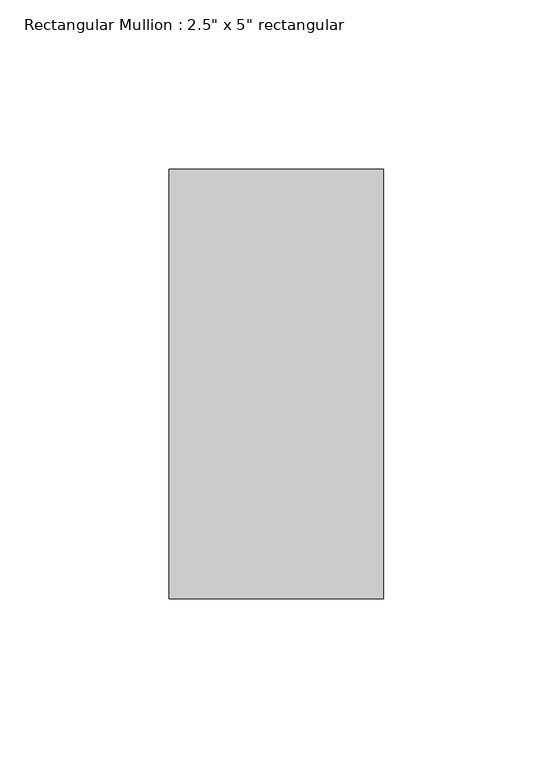
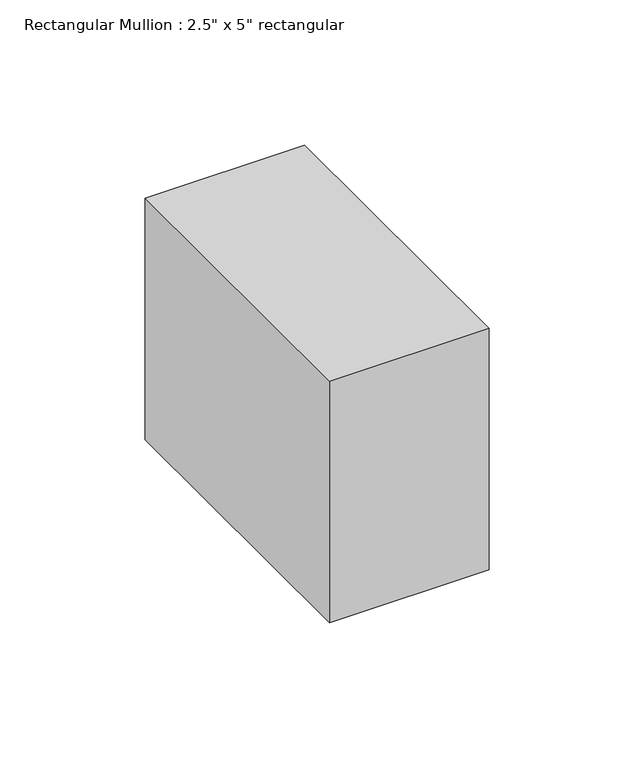
"""IFC4 building model written with IfcOpenShell, lengths in millimetres: member geometry."""

from ifc_helpers import new_model, si_unit, frame, origin, place, context, project, spatial, polyline, outline, extrude, source, transform, mapped, element, save


def member_4d11dfbc(model_context):
    return source(origin(), model_context, "Body", "SweptSolid", [
        extrude(outline(polyline([(0.0, 63.5), (0.0, -63.5), (-63.5, -63.5), (-63.5, 63.5), (0.0, 63.5)])), frame((0.0, 0.0, -101.5332841), z_axis=(0.0, 0.0, 1.0), x_axis=(1.0, 0.0, 0.0)), (0.0, 0.0, 1.0), 101.5332841),
    ])


if __name__ == "__main__":
    model = new_model("IFC4")
    model_context = context("Model", 3, world=origin())
    ifc_project = project(units=[si_unit("LENGTHUNIT", "METRE", prefix="MILLI")], contexts=[model_context])
    site = spatial("IfcSite", under=ifc_project)
    building = spatial("IfcBuilding", under=site)
    placement = place(None, origin())
    member_shape = member_4d11dfbc(model_context)
    element("IfcMember", 1, ObjectType="Rectangular Mullion : 2.5\" x 5\" rectangular", at=placement, inside=building, context=model_context, shape_type="MappedRepresentation", body=[
        mapped(member_shape, transform((0.0, 0.0, 0.0), x_axis=(1.0, 0.0, 0.0), y_axis=(0.0, 1.0, 0.0), z_axis=(0.0, 0.0, 1.0))),
    ])
    save(model, "model.ifc")

# Revit data of these elements
# Type "Rectangular Mullion : 2.5\" x 5\" rectangular"
#   built-in parameter 1007304 = 0.416667 (stored number, unit not read)
#   built-in parameter 1007301 = 0.104167 (stored number, unit not read)
#   built-in parameter 1007300 = 0.104167 (stored number, unit not read)
# Element 1 (IfcMember, "Rectangular Mullion : 2.5\" x 5\" rectangular")
#   Materials on its faces: "Aluminum"
# Materials
#   "Aluminum": class "Metal", colour RGB 247 247 247, transparency 0, Description = "Aluminum 6061", Cost = 0
